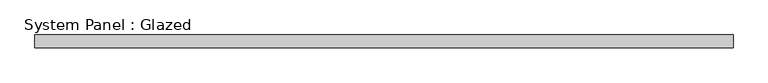
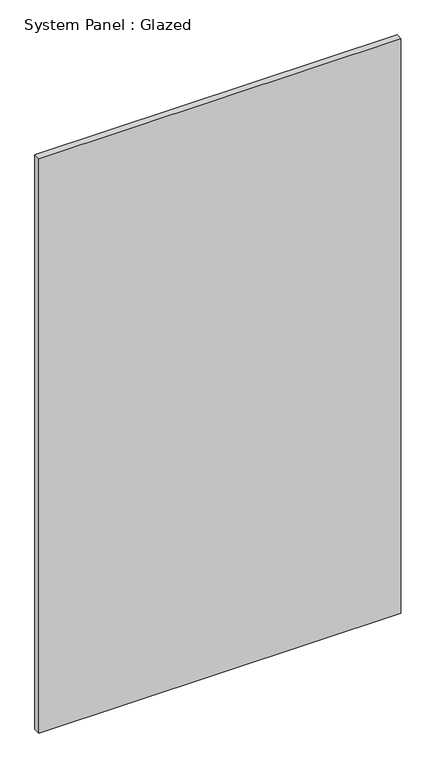
"""IFC4 building model written with IfcOpenShell, lengths in millimetres: plate geometry, System Panel : Glazed."""

from ifc_helpers import new_model, si_unit, origin, origin_with_axes, place, context, project, spatial, polyline, outline, extrude, source, transform, mapped, element, save


def system_panel_glazed_7a129d22(model_context):
    return source(origin(), model_context, "Body", "SweptSolid", [
        extrude(outline(polyline([(698.6142406, -44.45), (-698.6142406, -44.45), (-698.6142406, -19.05), (698.6142406, -19.05), (698.6142406, -44.45)])), origin_with_axes(), (0.0, 0.0, 1.0), 2343.15),
    ])


if __name__ == "__main__":
    model = new_model("IFC4")
    model_context = context("Model", 3, world=origin())
    ifc_project = project(units=[si_unit("LENGTHUNIT", "METRE", prefix="MILLI")], contexts=[model_context])
    site = spatial("IfcSite", under=ifc_project)
    building = spatial("IfcBuilding", under=site)
    placement = place(None, origin())
    system_panel_glazed_shape = system_panel_glazed_7a129d22(model_context)
    element("IfcPlate", 1, ObjectType="System Panel : Glazed", at=placement, inside=building, context=model_context, shape_type="MappedRepresentation", body=[
        mapped(system_panel_glazed_shape, transform((0.0, 0.0, 0.0), x_axis=(1.0, 0.0, 0.0), y_axis=(0.0, 1.0, 0.0), z_axis=(0.0, 0.0, 1.0))),
    ])
    save(model, "model.ifc")

# Revit data of these elements
# Type "System Panel : Glazed"
#   Construction Type Id = "GSP4R"
#   Analytic Construction = "1/8 in Pilkington single glazing"
#   Visual Light Transmittance = 0.9
#   Solar Heat Gain Coefficient = 0.86
#   Heat Transfer Coefficient (U) = 1.18115 BTU/(h·ft²·°F)
#   Define Thermal Properties by = 1
# Element 1 (IfcPlate, "System Panel : Glazed")
#   Materials on its faces: "glass panel 223"
# Materials
#   "glass panel 223": class "Generic", colour RGB 120 120 120, transparency 0, Cost = 0
